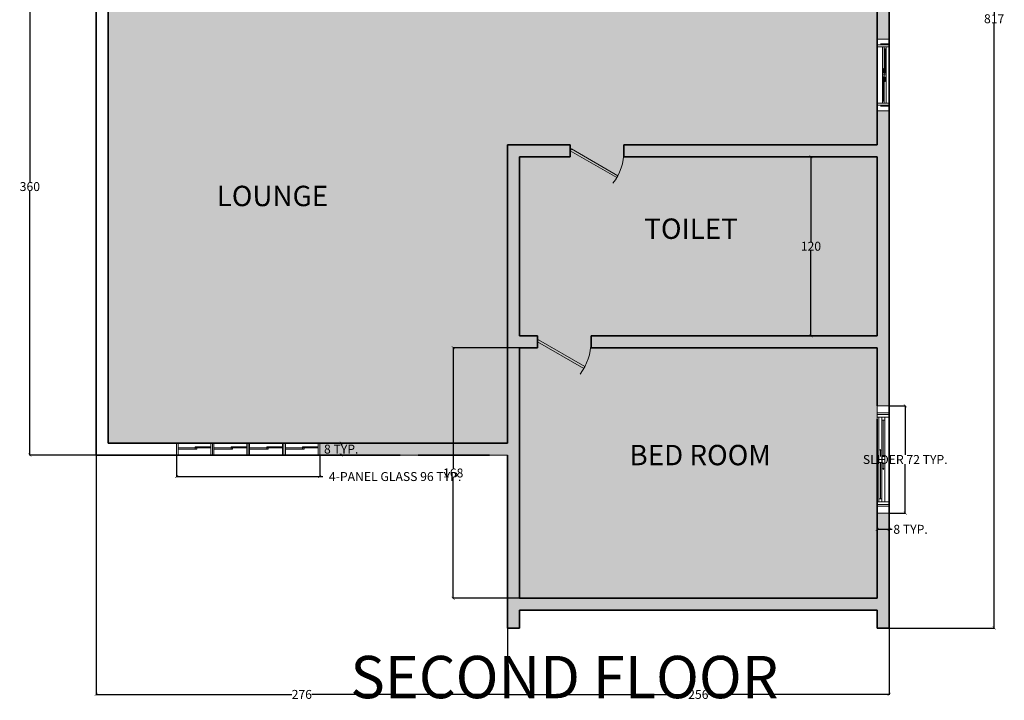
# Model space of a CAD drawing. Units: inches. Extents: x 1704 to 6393, y -157 to 1172.
# Tile 120 of 122: x 5732 to 6393, y -80 to 376. Entities that reach past the tile are written whole.
import ezdxf

# ---------------------------------------------------------------- set-up
doc = ezdxf.new("R2010")
doc.units = ezdxf.units.IN
doc.header["$MEASUREMENT"] = 0
doc.linetypes.add('ACAD_ISO02W100', pattern=[15, 12, -3])
for name, color, linetype, lineweight in [('A-ANNO-DIMS', 7, 'Continuous', 13), ('A-ANNO-TEXT', 7, 'Continuous', 25), ('A-AREA-IDEN', 7, 'Continuous', 18), ('A-WALL-OVHD', 8, 'ACAD_ISO02W100', 13), ('A-WALL-PATT', 7, 'Continuous', 13), ('DOORS', 160, 'Continuous', 18), ('GLASS PANEL FASADE', 4, 'Continuous', 18), ('WALLS', 7, 'Continuous', 35), ('WINDOWS', 2, 'Continuous', 18)]:
    doc.layers.add(name, color=color, linetype=linetype, lineweight=lineweight)
doc.layers.add('A-FLOR-PATT', color=7, linetype='Continuous', lineweight=13, true_color=0xf2f2f2)
doc.styles.get("Standard").update_dxf_attribs({"font": 'arial.ttf'})
doc.dimstyles.get("Standard").update_dxf_attribs({"dimtxt": 6, "dimasz": 2, "dimexe": 0.18, "dimexo": 0.0625, "dimgap": 0.09, "dimtad": 0, "dimtih": 1, "dimtoh": 1, "dimdec": 1, "dimzin": 0, "dimdsep": 46, "dimlunit": 3, "dimtxsty": 'Standard', "dimblk": 'ARCHTICK', "dimcen": 0.09, "dimadec": 0, "dimazin": 0, "dimtfac": 1, "dimtdec": 1, "dimtofl": 0, "dimtmove": 0, "dimatfit": 3, "dimfxl": 1, "dimtolj": 1, "dimtzin": 0, "dimarcsym": 0})

# ---------------------------------------------------------------- blocks, each defined once
blk = doc.blocks.new('Door - Left Hung 36 in.')
blk.add_lwpolyline([(0.75, -1.3), (0, 0), (31.18, 18), (31.93, 16.7)], close=True)
blk.add_arc((0, 0), 36, 0, 37.31013)
blk = doc.blocks.new('WIN-SLIDER-48')
for p, q in [((3.83, 8), (0, 8)), ((5.13, 8), (42.87, 8)), ((44.17, 8), (48, 8)), ((3.18, 5.86), (3.18, 0.65)), ((24, 1.95), (5.13, 1.95)), ((6.43, 4.55), (22.7, 4.55)), ((6.43, 3.9), (22.7, 3.9)), ((6.43, 3.25), (22.7, 3.25)), ((22.7, 2.6), (19.9, 2.6)), ((24, 4.55), (42.87, 4.55)), ((25.3, 3.9), (28.1, 3.9)), ((25.3, 3.25), (41.56, 3.25)), ((25.3, 2.6), (41.56, 2.6)), ((25.3, 1.95), (41.56, 1.95)), ((44.82, 5.86), (44.82, 0.65)), ((3.83, 0), (0, 0)), ((5.13, 0), (42.87, 0)), ((44.17, 0), (48, 0))]:
    blk.add_line(p, q)
for points in [[(5.13, 0), (3.83, 0), (3.83, 8), (5.13, 8)], [(42.87, 0), (44.17, 0), (44.17, 8), (42.87, 8)], [(5.13, 3.25), (6.43, 3.25), (6.43, 4.55), (5.13, 4.55)], [(19.57, 2.6), (19.9, 2.8), (19.9, 2.41)], [(22.7, 3.25), (24, 3.25), (24, 4.55), (22.7, 4.55)], [(24, 1.95), (25.3, 1.95), (25.3, 3.25), (24, 3.25)], [(28.43, 3.9), (28.1, 4.1), (28.1, 3.71)], [(41.56, 1.95), (42.87, 1.95), (42.87, 3.25), (41.56, 3.25)]]:
    blk.add_lwpolyline(points, close=True)
blk = doc.blocks.new('WIN-SLIDER-72')
for p, q in [((0, 72), (0, 0)), ((0, 72), (8, 72)), ((0, 67.23), (8, 67.23)), ((8, 66.25), (8, 72)), ((1.17, 36), (1.17, 64.3)), ((3.12, 37.95), (3.12, 62.35)), ((4.1, 37.95), (4.1, 62.35)), ((5.07, 37.95), (5.07, 62.35)), ((8, 7.7), (8, 64.3)), ((2.14, 37.95), (2.14, 42.14)), ((1.17, 9.65), (1.17, 34.05)), ((2.14, 9.65), (2.14, 34.05)), ((3.12, 9.65), (3.12, 34.05)), ((4.1, 34.05), (4.1, 29.86)), ((5.07, 36), (5.07, 7.7)), ((0, 4.77), (8, 4.77)), ((8, 5.75), (8, 0)), ((0, 0), (8, 0))]:
    blk.add_line(p, q)
for points in [[(8, 64.3), (8, 66.25), (0, 66.25), (0, 64.3)], [(5.07, 62.35), (5.07, 64.3), (3.12, 64.3), (3.12, 62.35)], [(2.14, 42.65), (1.85, 42.14), (2.44, 42.14)], [(3.12, 34.05), (3.12, 36), (1.17, 36), (1.17, 34.05)], [(5.07, 36), (5.07, 37.95), (3.12, 37.95), (3.12, 36)], [(4.1, 29.35), (3.8, 29.86), (4.39, 29.86)], [(8, 7.7), (8, 5.75), (0, 5.75), (0, 7.7)], [(3.12, 7.7), (3.12, 9.65), (1.17, 9.65), (1.17, 7.7)]]:
    blk.add_lwpolyline(points, close=True)
blk = doc.blocks.new('GLAZ-FOUR-PANEL-96')
for p, q in [((96, 8), (0, 8)), ((0, 8), (0, 0)), ((1, 8), (1, 0)), ((23, 8), (23, 0)), ((24, 8), (24, 0)), ((25, 8), (25, 0)), ((47, 8), (47, 0)), ((48, 8), (48, 0)), ((49, 8), (49, 0)), ((71, 8), (71, 0)), ((72, 8), (72, 0)), ((73, 8), (73, 0)), ((95, 0), (95, 8)), ((96, 0), (96, 8)), ((12.51, 4.77), (1, 4.77)), ((1, 4), (12.51, 4)), ((12.51, 4.77), (12.51, 5.55)), ((12.51, 5.55), (23, 5.55)), ((12.51, 4), (12.51, 4.77)), ((12.51, 4.77), (23, 4.77)), ((12.51, 4), (13.51, 4)), ((13.51, 4), (13.51, 5.55)), ((36.51, 4.77), (25, 4.77)), ((25, 4), (36.51, 4)), ((36.51, 4.77), (36.51, 5.55)), ((36.51, 5.55), (47, 5.55)), ((36.51, 4), (36.51, 4.77)), ((36.51, 4.77), (47, 4.77)), ((36.51, 4), (37.51, 4)), ((37.51, 4), (37.51, 5.55)), ((60.51, 4.77), (49, 4.77)), ((49, 4), (60.51, 4)), ((60.51, 4.77), (60.51, 5.55)), ((60.51, 5.55), (71, 5.55)), ((60.51, 4), (60.51, 4.77)), ((60.51, 4.77), (71, 4.77)), ((60.51, 4), (61.51, 4)), ((61.51, 4), (61.51, 5.55)), ((84.51, 4.77), (73, 4.77)), ((73, 4), (84.51, 4)), ((84.51, 4.77), (84.51, 5.55)), ((84.51, 5.55), (95, 5.55)), ((84.51, 4), (84.51, 4.77)), ((84.51, 4.77), (95, 4.77)), ((84.51, 4), (85.51, 4)), ((85.51, 4), (85.51, 5.55)), ((0, 0), (96, 0))]:
    blk.add_line(p, q)
blk = doc.blocks.new('_ArchTick')
at = {"color": 0, "linetype": 'ByBlock', "const_width": 0.15}
blk.add_lwpolyline([(-0.5, -0.5), (0.5, 0.5)], dxfattribs=at)
blk = doc.blocks.new('*D40')
at = {"layer": 'A-ANNO-DIMS', "color": 0, "lineweight": -2, "transparency": 16777216}
for p, q in [((6315.65, 117.52), (6326.57, 117.52)), ((6326.39, 117.52), (6326.39, 84.72)), ((6326.39, 45.52), (6326.39, 78.33)), ((6315.65, 45.52), (6326.57, 45.52))]:
    blk.add_line(p, q, dxfattribs=at)
at = {"layer": 'Defpoints', "color": 0, "lineweight": -3, "transparency": 16777216}
for p in [(6315.59, 117.52), (6326.39, 117.52), (6315.59, 45.52)]:
    blk.add_point(p, dxfattribs=at)
at = {"layer": 'A-ANNO-DIMS', "color": 0, "lineweight": -2, "transparency": 16777216, "xscale": 2, "yscale": 2, "zscale": 2}
for p, rotation in [((6326.39, 117.52), 90), ((6326.39, 45.52), 270)]:
    blk.add_blockref('_ArchTick', p, dxfattribs=dict(at, rotation=rotation))
at = {"layer": 'A-ANNO-DIMS', "color": 0, "transparency": 16777216, "insert": (6326.39, 81.52), "char_height": 6, "attachment_point": 5}
blk.add_mtext('\\A1;SLIDER 72 TYP.', dxfattribs=at)
blk = doc.blocks.new('*D41')
at = {"layer": 'A-ANNO-DIMS', "color": 0, "lineweight": -2, "transparency": 16777216}
for p, q in [((6307.59, 45.46), (6307.59, 34.54)), ((6315.59, 45.46), (6315.59, 34.54)), ((6307.59, 34.72), (6315.59, 34.72)), ((6315.59, 34.72), (6317.59, 34.72))]:
    blk.add_line(p, q, dxfattribs=at)
at = {"layer": 'Defpoints', "color": 0, "lineweight": -3, "transparency": 16777216}
for p in [(6307.59, 45.52), (6315.59, 45.52), (6315.59, 34.72)]:
    blk.add_point(p, dxfattribs=at)
at = {"layer": 'A-ANNO-DIMS', "color": 0, "lineweight": -2, "transparency": 16777216, "xscale": 2, "yscale": 2, "zscale": 2, "rotation": 180}
blk.add_blockref('_ArchTick', (6307.59, 34.72), dxfattribs=at)
at = {"layer": 'A-ANNO-DIMS', "color": 0, "lineweight": -2, "transparency": 16777216, "xscale": 2, "yscale": 2, "zscale": 2}
blk.add_blockref('_ArchTick', (6315.59, 34.72), dxfattribs=at)
at = {"layer": 'A-ANNO-DIMS', "color": 0, "transparency": 16777216, "insert": (6329.96, 34.72), "char_height": 6, "attachment_point": 5}
blk.add_mtext('\\A1;8 TYP.', dxfattribs=at)
blk = doc.blocks.new('*D46')
at = {"layer": 'A-ANNO-DIMS', "color": 0, "lineweight": -2, "transparency": 16777216}
for p, q in [((5837.6, 84.42), (5837.6, 69.9)), ((5933.6, 84.42), (5933.6, 69.9)), ((5837.6, 70.08), (5933.6, 70.08)), ((5933.6, 70.08), (5935.6, 70.08))]:
    blk.add_line(p, q, dxfattribs=at)
at = {"layer": 'Defpoints', "color": 0, "lineweight": -3, "transparency": 16777216}
for p in [(5837.6, 84.48), (5933.6, 84.48), (5933.6, 70.08)]:
    blk.add_point(p, dxfattribs=at)
at = {"layer": 'A-ANNO-DIMS', "color": 0, "lineweight": -2, "transparency": 16777216, "xscale": 2, "yscale": 2, "zscale": 2, "rotation": 180}
blk.add_blockref('_ArchTick', (5837.6, 70.08), dxfattribs=at)
at = {"layer": 'A-ANNO-DIMS', "color": 0, "lineweight": -2, "transparency": 16777216, "xscale": 2, "yscale": 2, "zscale": 2}
blk.add_blockref('_ArchTick', (5933.6, 70.08), dxfattribs=at)
at = {"layer": 'A-ANNO-DIMS', "color": 0, "transparency": 16777216, "insert": (5984.19, 70.08), "char_height": 6, "attachment_point": 5}
blk.add_mtext('\\A1;4-PANEL GLASS 96 TYP.', dxfattribs=at)
blk = doc.blocks.new('*D47')
at = {"layer": 'A-ANNO-DIMS', "color": 0, "lineweight": -2, "transparency": 16777216}
for p, q in [((5933.66, 92.48), (5948.18, 92.48)), ((5948, 92.48), (5948, 91.63)), ((5933.66, 84.48), (5948.18, 84.48)), ((5948, 84.48), (5948, 85.32))]:
    blk.add_line(p, q, dxfattribs=at)
at = {"layer": 'Defpoints', "color": 0, "lineweight": -3, "transparency": 16777216}
for p in [(5933.6, 92.48), (5948, 92.48), (5933.6, 84.48)]:
    blk.add_point(p, dxfattribs=at)
at = {"layer": 'A-ANNO-DIMS', "color": 0, "lineweight": -2, "transparency": 16777216, "xscale": 2, "yscale": 2, "zscale": 2}
for p, rotation in [((5948, 92.48), 90), ((5948, 84.48), 270)]:
    blk.add_blockref('_ArchTick', p, dxfattribs=dict(at, rotation=rotation))
at = {"layer": 'A-ANNO-DIMS', "color": 0, "transparency": 16777216, "insert": (5948, 88.48), "char_height": 6, "attachment_point": 5}
blk.add_mtext('\\A1;8 TYP.', dxfattribs=at)
blk = doc.blocks.new('*D120')
at = {"layer": 'A-ANNO-DIMS', "color": 0, "lineweight": -2, "transparency": 16777216}
for p, q in [((6315.65, 785.48), (6386.22, 785.48)), ((6386.04, 785.48), (6386.04, 380.13)), ((6386.04, -31.52), (6386.04, 373.82)), ((6315.65, -31.52), (6386.22, -31.52))]:
    blk.add_line(p, q, dxfattribs=at)
at = {"layer": 'Defpoints', "color": 0, "lineweight": -3, "transparency": 16777216}
for p in [(6315.59, 785.48), (6315.59, -31.52), (6386.04, -31.52)]:
    blk.add_point(p, dxfattribs=at)
at = {"layer": 'A-ANNO-DIMS', "color": 0, "lineweight": -2, "transparency": 16777216, "xscale": 2, "yscale": 2, "zscale": 2}
for p, rotation in [((6386.04, 785.48), 90), ((6386.04, -31.52), 270)]:
    blk.add_blockref('_ArchTick', p, dxfattribs=dict(at, rotation=rotation))
at = {"layer": 'A-ANNO-DIMS', "color": 0, "transparency": 16777216, "insert": (6386.04, 376.98), "char_height": 6, "attachment_point": 5}
blk.add_mtext('\\A1;817', dxfattribs=at)
blk = doc.blocks.new('*D121')
at = {"layer": 'A-ANNO-DIMS', "color": 0, "lineweight": -2, "transparency": 16777216}
for p, q in [((5783.6, 84.42), (5783.6, -76.15)), ((6059.59, 84.42), (6059.59, -76.15)), ((5783.6, -75.97), (5914.83, -75.97)), ((6059.59, -75.97), (5928.36, -75.97))]:
    blk.add_line(p, q, dxfattribs=at)
at = {"layer": 'Defpoints', "color": 0, "lineweight": -3, "transparency": 16777216}
for p in [(5783.6, 84.48), (6059.59, 84.48), (6059.59, -75.97)]:
    blk.add_point(p, dxfattribs=at)
at = {"layer": 'A-ANNO-DIMS', "color": 0, "lineweight": -2, "transparency": 16777216, "xscale": 2, "yscale": 2, "zscale": 2, "rotation": 180}
blk.add_blockref('_ArchTick', (5783.6, -75.97), dxfattribs=at)
at = {"layer": 'A-ANNO-DIMS', "color": 0, "lineweight": -2, "transparency": 16777216, "xscale": 2, "yscale": 2, "zscale": 2}
blk.add_blockref('_ArchTick', (6059.59, -75.97), dxfattribs=at)
at = {"layer": 'A-ANNO-DIMS', "color": 0, "transparency": 16777216, "insert": (5921.6, -75.97), "char_height": 6, "attachment_point": 5}
blk.add_mtext('\\A1;276', dxfattribs=at)
blk = doc.blocks.new('*D122')
at = {"layer": 'A-ANNO-DIMS', "color": 0, "lineweight": -2, "transparency": 16777216}
for p, q in [((6059.59, -31.58), (6059.59, -76.15)), ((6315.59, -31.58), (6315.59, -76.15)), ((6059.59, -75.97), (6180.82, -75.97)), ((6315.59, -75.97), (6194.36, -75.97))]:
    blk.add_line(p, q, dxfattribs=at)
at = {"layer": 'Defpoints', "color": 0, "lineweight": -3, "transparency": 16777216}
for p in [(6059.59, -31.52), (6315.59, -31.52), (6315.59, -75.97)]:
    blk.add_point(p, dxfattribs=at)
at = {"layer": 'A-ANNO-DIMS', "color": 0, "lineweight": -2, "transparency": 16777216, "xscale": 2, "yscale": 2, "zscale": 2, "rotation": 180}
blk.add_blockref('_ArchTick', (6059.59, -75.97), dxfattribs=at)
at = {"layer": 'A-ANNO-DIMS', "color": 0, "lineweight": -2, "transparency": 16777216, "xscale": 2, "yscale": 2, "zscale": 2}
blk.add_blockref('_ArchTick', (6315.59, -75.97), dxfattribs=at)
at = {"layer": 'A-ANNO-DIMS', "color": 0, "transparency": 16777216, "insert": (6187.59, -75.97), "char_height": 6, "attachment_point": 5}
blk.add_mtext('\\A1;256', dxfattribs=at)
blk = doc.blocks.new('*D123')
at = {"layer": 'A-ANNO-DIMS', "color": 0, "lineweight": -2, "transparency": 16777216}
for p, q in [((5783.53, 444.48), (5738.96, 444.48)), ((5739.14, 444.48), (5739.14, 267.63)), ((5739.14, 84.48), (5739.14, 261.32)), ((5783.54, 84.48), (5738.96, 84.48))]:
    blk.add_line(p, q, dxfattribs=at)
at = {"layer": 'Defpoints', "color": 0, "lineweight": -3, "transparency": 16777216}
for p in [(5739.14, 444.48), (5783.59, 444.48), (5783.6, 84.48)]:
    blk.add_point(p, dxfattribs=at)
at = {"layer": 'A-ANNO-DIMS', "color": 0, "lineweight": -2, "transparency": 16777216, "xscale": 2, "yscale": 2, "zscale": 2}
for p, rotation in [((5739.14, 444.48), 90), ((5739.14, 84.48), 270)]:
    blk.add_blockref('_ArchTick', p, dxfattribs=dict(at, rotation=rotation))
at = {"layer": 'A-ANNO-DIMS', "color": 0, "transparency": 16777216, "insert": (5739.14, 264.48), "char_height": 6, "attachment_point": 5}
blk.add_mtext('\\A1;360', dxfattribs=at)
blk = doc.blocks.new('*D129')
at = {"layer": 'A-ANNO-DIMS', "color": 0, "lineweight": -2, "transparency": 16777216}
for p, q in [((6307.53, 284.48), (6262.96, 284.48)), ((6263.14, 284.48), (6263.14, 227.63)), ((6263.14, 164.48), (6263.14, 221.32)), ((6307.53, 164.48), (6262.96, 164.48))]:
    blk.add_line(p, q, dxfattribs=at)
at = {"layer": 'Defpoints', "color": 0, "lineweight": -3, "transparency": 16777216}
for p in [(6263.14, 284.48), (6307.59, 284.48), (6307.59, 164.48)]:
    blk.add_point(p, dxfattribs=at)
at = {"layer": 'A-ANNO-DIMS', "color": 0, "lineweight": -2, "transparency": 16777216, "xscale": 2, "yscale": 2, "zscale": 2}
for p, rotation in [((6263.14, 284.48), 90), ((6263.14, 164.48), 270)]:
    blk.add_blockref('_ArchTick', p, dxfattribs=dict(at, rotation=rotation))
at = {"layer": 'A-ANNO-DIMS', "color": 0, "transparency": 16777216, "insert": (6263.14, 224.48), "char_height": 6, "attachment_point": 5}
blk.add_mtext('\\A1;120', dxfattribs=at)
blk = doc.blocks.new('*D130')
at = {"layer": 'A-ANNO-DIMS', "color": 0, "lineweight": -2, "transparency": 16777216}
for p, q in [((6067.53, 156.48), (6022.96, 156.48)), ((6023.14, 156.48), (6023.14, 75.63)), ((6023.14, -11.52), (6023.14, 69.32)), ((6067.53, -11.52), (6022.96, -11.52))]:
    blk.add_line(p, q, dxfattribs=at)
at = {"layer": 'Defpoints', "color": 0, "lineweight": -3, "transparency": 16777216}
for p in [(6023.14, 156.48), (6067.59, 156.48), (6067.59, -11.52)]:
    blk.add_point(p, dxfattribs=at)
at = {"layer": 'A-ANNO-DIMS', "color": 0, "lineweight": -2, "transparency": 16777216, "xscale": 2, "yscale": 2, "zscale": 2}
for p, rotation in [((6023.14, 156.48), 90), ((6023.14, -11.52), 270)]:
    blk.add_blockref('_ArchTick', p, dxfattribs=dict(at, rotation=rotation))
at = {"layer": 'A-ANNO-DIMS', "color": 0, "transparency": 16777216, "insert": (6023.14, 72.48), "char_height": 6, "attachment_point": 5}
blk.add_mtext('\\A1;168', dxfattribs=at)

msp = doc.modelspace()

# ---------------------------------------------------------------- hatches: boundary and pattern name
at = {"layer": 'A-FLOR-PATT', "transparency": 33554559}
h = msp.add_hatch(color=256, dxfattribs=at)
h.dxf.hatch_style = 1
h.paths.add_polyline_path([(5979.59, 777.478), (5791.59, 777.478), (5791.59, 741.478), (5979.59, 741.478)], flags=17)
h.paths.add_polyline_path([(5979.59, 733.478), (5791.59, 733.478), (5791.59, 565.478), (5907.59, 565.478), (5907.59, 561.478), (5883.59, 561.478), (5883.59, 555.478), (5875.59, 555.478), (5875.59, 561.478), (5791.59, 561.478), (5791.59, 452.478), (5875.59, 452.478), (5875.59, 525.478), (5883.59, 525.478), (5883.59, 452.478), (5979.59, 452.478), (5979.59, 561.478), (5943.59, 561.478), (5943.59, 565.478), (5979.59, 565.478), (5987.59, 565.478), (5987.59, 444.478), (5791.59, 444.478), (5791.603, 92.478), (6059.59, 92.478), (6059.59, 292.478), (6101.682, 292.478), (6101.682, 284.478), (6067.59, 284.478), (6067.59, 164.478), (6079.59, 164.478), (6079.59, 156.478), (6067.59, 156.478), (6067.59, -11.522), (6307.59, -11.522), (6307.59, 108.478), (6307.59, 117.524), (6307.59, 156.478), (6115.59, 156.478), (6115.59, 164.478), (6307.59, 164.478), (6307.59, 236.478), (6307.59, 262.478), (6307.59, 284.478), (6137.682, 284.478), (6137.682, 292.478), (6307.59, 292.478), (6307.59, 428.478), (6068.59, 428.478), (6060.59, 428.478), (6060.59, 455.978), (6068.59, 455.978), (6068.59, 435.478), (6130.59, 435.478), (6130.59, 500.478), (6068.59, 500.478), (6068.59, 479.978), (6060.59, 479.978), (6060.59, 505.478), (6135.59, 505.478), (6135.59, 497.478), (6135.59, 436.478), (6183.59, 436.478), (6183.59, 454.978), (6187.59, 454.978), (6187.59, 436.478), (6262.788, 436.478), (6262.788, 497.478), (6187.59, 497.478), (6187.59, 478.978), (6183.59, 478.978), (6183.59, 497.478), (6159.59, 497.478), (6159.59, 505.478), (6161.98, 505.478), (6161.98, 549.478), (6137.98, 549.478), (6137.98, 555.478), (6077.98, 555.478), (6077.98, 557.478), (6077.98, 601.478), (6029.59, 601.478), (6029.59, 609.478), (6035.59, 609.478), (6207.59, 609.478), (6207.59, 641.478), (6211.59, 641.478), (6211.59, 609.478), (6223.59, 609.478), (6307.59, 609.478), (6307.59, 677.478), (6271.59, 677.478), (6271.59, 681.478), (6307.59, 681.478), (6307.59, 735.174), (6211.59, 735.174), (6211.59, 681.478), (6247.59, 681.478), (6247.59, 677.478), (6211.59, 677.478), (6207.59, 677.478), (6207.59, 777.478), (5987.59, 777.478), (5987.59, 609.478), (5993.59, 609.478), (5993.59, 601.478), (5979.59, 601.478)])
h.paths.add_polyline_path([(6307.59, 601.478), (6261.59, 601.478), (6261.59, 505.478), (6307.59, 505.478), (6307.59, 535.478)], flags=17)
h.paths.add_polyline_path([(6161.98, 601.478), (6138.98, 601.478), (6138.98, 557.478), (6161.98, 557.478)], flags=17)
h.paths.add_polyline_path([(6257.59, 601.478), (6242.98, 601.478), (6242.98, 557.478), (6257.59, 557.478)], flags=17)
h.paths.add_polyline_path([(6117.98, 601.478), (6108.98, 601.478), (6108.98, 557.478), (6117.98, 557.478)], flags=17)
h.paths.add_polyline_path([(6107.98, 601.478), (6098.98, 601.478), (6098.98, 557.478), (6107.98, 557.478)], flags=17)
h.paths.add_polyline_path([(6097.98, 601.478), (6088.98, 601.478), (6088.98, 557.478), (6097.98, 557.478)], flags=17)
h.paths.add_polyline_path([(6087.98, 601.478), (6078.98, 601.478), (6078.98, 557.478), (6087.98, 557.478)], flags=17)
h.paths.add_polyline_path([(6127.98, 601.478), (6118.98, 601.478), (6118.98, 557.478), (6127.98, 557.478)], flags=17)
h.paths.add_polyline_path([(6137.98, 601.478), (6128.98, 601.478), (6128.98, 557.478), (6137.98, 557.478)], flags=17)
h.paths.add_polyline_path([(6171.98, 601.478), (6162.98, 601.478), (6162.98, 557.478), (6171.98, 557.478)], flags=17)
h.paths.add_polyline_path([(6181.98, 601.478), (6172.98, 601.478), (6172.98, 557.478), (6181.98, 557.478)], flags=17)
h.paths.add_polyline_path([(6191.98, 601.478), (6182.98, 601.478), (6182.98, 557.478), (6191.98, 557.478)], flags=17)
h.paths.add_polyline_path([(6201.98, 601.478), (6192.98, 601.478), (6192.98, 557.478), (6201.98, 557.478)], flags=17)
h.paths.add_polyline_path([(6211.98, 601.478), (6202.98, 601.478), (6202.98, 557.478), (6211.98, 557.478)], flags=17)
h.paths.add_polyline_path([(6221.98, 601.478), (6212.98, 601.478), (6212.98, 557.478), (6221.98, 557.478)], flags=17)
h.paths.add_polyline_path([(6231.98, 601.478), (6222.98, 601.478), (6222.98, 557.478), (6231.98, 557.478)], flags=17)
h.paths.add_polyline_path([(6241.98, 601.478), (6232.98, 601.478), (6232.98, 557.478), (6241.98, 557.478)], flags=17)
h.paths.add_polyline_path([(6171.98, 549.478), (6162.98, 549.478), (6162.98, 505.478), (6171.98, 505.478)], flags=17)
h.paths.add_polyline_path([(6181.98, 549.478), (6172.98, 549.478), (6172.98, 505.478), (6181.98, 505.478)], flags=17)
h.paths.add_polyline_path([(6191.98, 549.478), (6182.98, 549.478), (6182.98, 505.478), (6191.98, 505.478)], flags=17)
h.paths.add_polyline_path([(6201.98, 549.478), (6192.98, 549.478), (6192.98, 505.478), (6201.98, 505.478)], flags=17)
h.paths.add_polyline_path([(6211.98, 549.478), (6202.98, 549.478), (6202.98, 505.478), (6211.98, 505.478)], flags=17)
h.paths.add_polyline_path([(6221.98, 549.478), (6212.98, 549.478), (6212.98, 505.478), (6221.98, 505.478)], flags=17)
h.paths.add_polyline_path([(6231.98, 549.478), (6222.98, 549.478), (6222.98, 505.478), (6231.98, 505.478)], flags=17)
h.paths.add_polyline_path([(6241.98, 549.478), (6232.98, 549.478), (6232.98, 505.478), (6241.98, 505.478)], flags=17)
h.paths.add_polyline_path([(6257.59, 549.478), (6242.98, 549.478), (6242.98, 505.478), (6257.59, 505.478)], flags=17)
at = {"layer": 'A-WALL-PATT', "transparency": 33554559}
h = msp.add_hatch(color=256, dxfattribs=at)
h.dxf.hatch_style = 1
h.paths.add_polyline_path([(6315.59, 785.478), (6047.299, 785.478), (6047.299, 777.478), (6207.59, 777.478), (6207.59, 677.478), (6211.59, 677.478), (6247.59, 677.478), (6247.59, 681.478), (6211.59, 681.478), (6211.59, 777.478), (6307.59, 777.478), (6307.59, 744.478), (6307.59, 677.478), (6307.59, 609.478), (6211.59, 609.478), (6211.59, 641.478), (6207.59, 641.478), (6207.59, 609.478), (6035.59, 609.478), (6029.59, 609.478), (6029.59, 601.478), (6257.59, 601.478), (6257.59, 505.478), (6159.59, 505.478), (6159.59, 497.478), (6183.59, 497.478), (6183.59, 478.978), (6187.59, 478.978), (6187.59, 497.478), (6307.59, 497.478), (6307.59, 436.478), (6187.59, 436.478), (6187.59, 454.978), (6183.59, 454.978), (6183.59, 436.478), (6135.59, 436.478), (6135.59, 497.478), (6135.59, 505.478), (6060.59, 505.478), (6060.59, 479.978), (6068.59, 479.978), (6068.59, 500.478), (6130.59, 500.478), (6130.59, 435.478), (6068.59, 435.478), (6068.59, 455.978), (6060.59, 455.978), (6060.59, 428.478), (6187.59, 428.478), (6307.59, 428.478), (6307.59, 385.478), (6307.59, 363.289), (6315.59, 363.289), (6315.59, 402.478), (6315.59, 404.478), (6315.59, 456.478), (6315.59, 458.478), (6315.59, 497.478), (6315.59, 505.478), (6307.59, 505.478), (6261.59, 505.478), (6261.59, 601.478), (6307.59, 601.478), (6307.59, 535.478), (6315.59, 535.478), (6315.59, 602.478), (6315.59, 606.478), (6315.59, 642.478), (6315.59, 644.478)])
h.paths.add_polyline_path([(5791.59, 561.478), (5875.59, 561.478), (5875.59, 555.478), (5883.59, 555.478), (5883.59, 561.478), (5907.59, 561.478), (5907.59, 565.478), (5791.59, 565.478), (5783.59, 565.478), (5783.59, 444.478), (5987.59, 444.478), (5987.59, 565.478), (5979.59, 565.478), (5943.59, 565.478), (5943.59, 561.478), (5979.59, 561.478), (5979.59, 452.478), (5883.59, 452.478), (5883.59, 525.478), (5875.59, 525.478), (5875.59, 452.478), (5791.59, 452.478)])
h = msp.add_hatch(color=256, dxfattribs=at)
h.dxf.hatch_style = 1
h.paths.add_polyline_path([(6067.59, 156.478), (6079.59, 156.478), (6079.59, 164.478), (6067.59, 164.478), (6067.59, 284.478), (6101.682, 284.478), (6101.682, 292.478), (6059.59, 292.478), (6059.59, 92.478), (5933.597, 92.478), (5933.597, 84.478), (5987.59, 84.478), (5999.59, 84.478), (6047.59, 84.478), (6059.59, 84.478), (6059.59, -19.522), (6059.59, -31.522), (6067.59, -31.522), (6067.59, -19.522), (6307.59, -19.522), (6307.59, -31.522), (6315.59, -31.522), (6315.59, -19.522), (6315.59, 45.524), (6307.59, 45.524), (6307.59, -11.522), (6067.59, -11.522)])
h.paths.add_polyline_path([(6315.59, 315.289), (6307.59, 315.289), (6307.59, 292.478), (6137.682, 292.478), (6137.682, 284.478), (6307.59, 284.478), (6307.59, 262.478), (6307.59, 236.478), (6307.59, 164.478), (6115.59, 164.478), (6115.59, 156.478), (6307.59, 156.478), (6307.59, 117.524), (6315.59, 117.524)])

# ---------------------------------------------------------------- linework, layer by layer
at = {"layer": 'A-WALL-OVHD'}
for p, q in [((5987.59, 92.478), (5999.59, 92.478)), ((5987.59, 84.478), (5999.59, 84.478)), ((6047.59, 84.478), (6059.59, 84.478))]:
    msp.add_line(p, q, dxfattribs=at)
at = {"layer": 'WALLS'}
for p, q in [((5783.59, 444.478), (5783.603, 92.478)), ((5791.59, 444.478), (5791.603, 92.478)), ((6307.59, 292.478), (6307.59, 428.478)), ((6315.59, 108.478), (6315.59, 402.478)), ((6059.59, 92.478), (6059.59, 292.478)), ((6101.682, 292.478), (6059.59, 292.478)), ((6101.682, 284.478), (6101.682, 292.478)), ((6307.59, 292.478), (6137.682, 292.478)), ((6137.682, 284.478), (6137.682, 292.478)), ((6067.59, 164.478), (6067.59, 284.478)), ((6101.682, 284.478), (6067.59, 284.478)), ((6307.59, 284.478), (6137.682, 284.478)), ((6307.59, 262.478), (6307.59, 284.478)), ((6307.59, 236.478), (6307.59, 262.478)), ((6307.59, 236.478), (6307.59, 254.478)), ((6307.59, 164.478), (6307.59, 236.478)), ((6307.59, 218.478), (6307.59, 228.478)), ((6079.59, 164.478), (6067.59, 164.478)), ((6079.59, 164.478), (6079.59, 156.478)), ((6307.59, 164.478), (6115.59, 164.478)), ((6115.59, 164.478), (6115.59, 156.478)), ((6067.59, -11.522), (6067.59, 156.478)), ((6079.59, 156.478), (6067.59, 156.478)), ((6307.59, 156.478), (6115.59, 156.478)), ((6307.59, 156.478), (6307.59, 117.524)), ((6307.59, -11.522), (6307.59, 108.478)), ((6315.59, -19.522), (6315.59, 108.478)), ((5783.603, 84.478), (5783.603, 92.478)), ((6059.59, 92.478), (5791.603, 92.478)), ((5987.59, 84.478), (5783.603, 84.478)), ((5999.59, 84.478), (6047.59, 84.478)), ((6059.59, -19.522), (6059.59, 84.478)), ((6307.59, -11.522), (6067.59, -11.522)), ((6059.59, -19.522), (6059.59, -31.522)), ((6307.59, -19.522), (6067.59, -19.522)), ((6067.59, -31.522), (6067.59, -19.522)), ((6307.59, -19.522), (6307.59, -31.522)), ((6315.59, -19.522), (6315.59, -31.522)), ((6059.59, -31.522), (6067.59, -31.522)), ((6315.59, -31.522), (6307.59, -31.522))]:
    msp.add_line(p, q, dxfattribs=at)
at = {"layer": 'WINDOWS'}
for p, q in [((6315.59, 363.289), (6307.59, 363.289)), ((6315.59, 315.289), (6307.59, 315.289))]:
    msp.add_line(p, q, dxfattribs=at)

# ---------------------------------------------------------------- block references
at = {"layer": 'DOORS', "xscale": -1, "rotation": 180}
for p in [(6101.682, 288.478), (6079.59, 160.478)]:
    msp.add_blockref('Door - Left Hung 36 in.', p, dxfattribs=at)
at = {"layer": 'GLASS PANEL FASADE'}
msp.add_blockref('GLAZ-FOUR-PANEL-96', (5837.597, 84.478), dxfattribs=at)
at = {"layer": 'WINDOWS', "rotation": 90.00000000000081}
msp.add_blockref('WIN-SLIDER-48', (6315.59, 315.29), dxfattribs=at)
at = {"layer": 'WINDOWS'}
msp.add_blockref('WIN-SLIDER-72', (6307.591, 45.524), dxfattribs=at)

# ---------------------------------------------------------------- texts
at = {"layer": 'A-ANNO-TEXT'}
msp.add_text('SECOND FLOOR', height=28.38733, dxfattribs=at).set_placement((5954.194, -78.538))
at = {"layer": 'A-AREA-IDEN'}
for s, p in [('LOUNGE', (5864.504, 251.352)), ('TOILET', (6151.33, 229.405)), (' BED ROOM', (6137.198, 77.651))]:
    msp.add_text(s, height=13.6672, dxfattribs=at).set_placement(p)

# ---------------------------------------------------------------- dimensions: what is measured, and where the dimension line sits
at = {"layer": 'A-ANNO-DIMS'}
for base, p1, p2, picture, middle in [((6386.04, -31.522), (6315.59, 785.478), (6315.59, -31.522), '*D120', (6386.04, 376.978)), ((5739.14, 444.478), (5783.603, 84.478), (5783.59, 444.478), '*D123', (5739.14, 264.478)), ((6263.14, 284.478), (6307.59, 164.478), (6307.59, 284.478), '*D129', (6263.14, 224.478)), ((6023.14, 156.478), (6067.59, -11.522), (6067.59, 156.478), '*D130', (6023.14, 72.478))]:
    dim = msp.add_linear_dim(base=base, p1=p1, p2=p2, angle=90, dimstyle='Standard', override={"dimdec": 0, "dimlfac": 1, "dimrnd": 0, "dimzin": 0, "dimdsep": 46, "dimlunit": 2}, dxfattribs=at)
    dim.commit()
    dim.dimension.update_dxf_attribs({"geometry": picture, "text_midpoint": middle})
for base, p1, p2, text, picture, middle in [((6326.39, 117.524), (6315.59, 45.524), (6315.59, 117.524), 'SLIDER <> TYP.', '*D40', (6326.39, 81.524)), ((5947.997, 92.478), (5933.597, 84.478), (5933.597, 92.478), '<> TYP.', '*D47', (5947.997, 88.478))]:
    dim = msp.add_linear_dim(base=base, p1=p1, p2=p2, angle=90, text=text, dimstyle='Standard', override={"dimdec": 0, "dimlfac": 1, "dimrnd": 0, "dimzin": 0, "dimdsep": 46, "dimlunit": 2}, dxfattribs=at)
    dim.commit()
    dim.dimension.update_dxf_attribs({"geometry": picture, "text_midpoint": middle})
for base, p1, p2, text, picture, middle in [((5933.597, 70.078), (5837.597, 84.478), (5933.597, 84.478), '4-PANEL GLASS <> TYP.', '*D46', (5984.186, 70.078)), ((6315.59, 34.724), (6307.59, 45.524), (6315.59, 45.524), '<> TYP.', '*D41', (6329.956, 34.724))]:
    dim = msp.add_linear_dim(base=base, p1=p1, p2=p2, text=text, dimstyle='Standard', override={"dimdec": 0, "dimlfac": 1, "dimrnd": 0, "dimzin": 0, "dimdsep": 46, "dimlunit": 2}, dxfattribs=at)
    dim.commit()
    dim.dimension.update_dxf_attribs({"geometry": picture, "text_midpoint": middle})
for base, p1, p2, picture, middle in [((6059.59, -75.972), (5783.603, 84.478), (6059.59, 84.478), '*D121', (5921.597, -75.972)), ((6315.59, -75.972), (6059.59, -31.522), (6315.59, -31.522), '*D122', (6187.59, -75.972))]:
    dim = msp.add_linear_dim(base=base, p1=p1, p2=p2, dimstyle='Standard', override={"dimdec": 0, "dimlfac": 1, "dimrnd": 0, "dimzin": 0, "dimdsep": 46, "dimlunit": 2}, dxfattribs=at)
    dim.commit()
    dim.dimension.update_dxf_attribs({"geometry": picture, "text_midpoint": middle})

doc.saveas('drawing.dxf')
